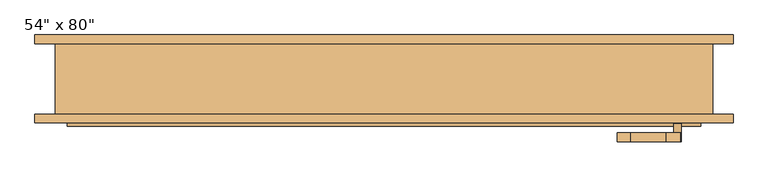
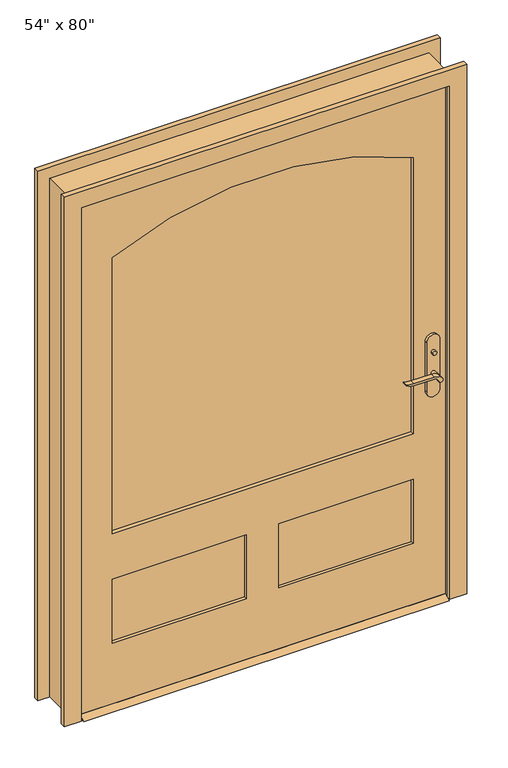
"""IFC4 building model written with IfcOpenShell, lengths in millimetres: door geometry."""

from ifc_helpers import new_model, si_unit, point, frame, frame_2d, origin, place, context, project, spatial, polyline, circle_curve, trimmed, segment, composite_curve, outline, extrude, faceted_brep, source, transform, mapped, element, save


def door_483975e0(model_context):
    return source(origin(), model_context, "Body", "SolidModel", [
        extrude(outline(polyline([(-38.1, 12.7), (-12.7, 0.0), (-98.425, 0.0), (-73.025, 12.7), (-38.1, 12.7)])), frame((-685.8, 0.0, 0.0), z_axis=(1.0, 0.0, 0.0), x_axis=(0.0, 1.0, 0.0)), (0.0, 0.0, 1.0), 1371.6),
        extrude(outline(polyline([(640.0, -18.1), (640.0, -28.1), (630.0, -28.1), (630.0, -18.1), (640.0, -18.1)])), frame((0.0, 0.0, 981.9), z_axis=(0.0, 0.0, 1.0), x_axis=(1.0, 0.0, 0.0)), (0.0, 0.0, 1.0), 30.0),
        extrude(outline(composite_curve([segment(trimmed(circle_curve(frame_2d((996.9, 635.0)), 8.0), [point((996.9, 627.0))], [point((996.9, 643.0))], False, "CARTESIAN"), True, "CONTINUOUS"), segment(trimmed(circle_curve(frame_2d((996.9, 635.0)), 8.0), [point((996.9, 643.0))], [point((996.9, 627.0))], False, "CARTESIAN"), True, "CONTINUOUS")], self_intersect=False)), frame((0.0, -93.025, 0.0), z_axis=(0.0, 1.0, 0.0), x_axis=(0.0, 0.0, 1.0)), (0.0, 0.0, 1.0), 10.0),
        extrude(outline(composite_curve([segment(trimmed(circle_curve(frame_2d((897.1555521, 611.3324871)), 37.2832219), [point((919.0523287, 641.5081363))], [point((934.4, 609.6325667))], False, "CARTESIAN"), True, "CONTINUOUS"), segment(polyline([(934.4, 609.6325667), (934.4, 533.3564091)]), True, "CONTINUOUS"), segment(trimmed(circle_curve(frame_2d((1017.6850638, 533.4227909)), 83.2850902), [point((934.4, 533.3564091))], [point((939.4, 505.0))], True, "CARTESIAN"), True, "CONTINUOUS"), segment(polyline([(939.4, 505.0), (936.6135558, 505.0)]), True, "CONTINUOUS"), segment(trimmed(circle_curve(frame_2d((986.6709207, 536.9396612)), 59.3791355), [point((936.6135558, 505.0))], [point((927.4, 533.3564091))], False, "CARTESIAN"), True, "CONTINUOUS"), segment(polyline([(927.4, 533.3564091), (927.4, 609.6138099)]), True, "CONTINUOUS"), segment(trimmed(circle_curve(frame_2d((909.2738613, 609.6138099)), 18.1261387), [point((927.4, 609.6138099))], [point((914.4, 627.0))], True, "CARTESIAN"), True, "CONTINUOUS"), segment(trimmed(circle_curve(frame_2d((914.4, 635.0)), 8.0), [point((914.4, 627.0))], [point((919.0523287, 641.5081363))], False, "CARTESIAN"), True, "CONTINUOUS")], self_intersect=False)), frame((0.0, 1.9, 0.0), z_axis=(0.0, 1.0, 0.0), x_axis=(0.0, 0.0, 1.0)), (0.0, 0.0, 1.0), 20.0),
        extrude(outline(composite_curve([segment(trimmed(circle_curve(frame_2d((914.4, 635.0)), 8.0), [point((914.3999903, 627.0))], [point((919.0523287, 641.5081363))], False, "CARTESIAN"), True, "CONTINUOUS"), segment(trimmed(circle_curve(frame_2d((897.1555521, 611.3324871)), 37.2832219), [point((919.0523287, 641.5081363))], [point((934.4, 609.6325667))], False, "CARTESIAN"), True, "CONTINUOUS"), segment(polyline([(934.4, 609.6325667), (934.4, 533.3564091)]), True, "CONTINUOUS"), segment(trimmed(circle_curve(frame_2d((1017.6850638, 533.4227909)), 83.2850902), [point((934.4, 533.3564091))], [point((939.4, 505.0))], True, "CARTESIAN"), True, "CONTINUOUS"), segment(polyline([(939.4, 505.0), (936.6135558, 505.0)]), True, "CONTINUOUS"), segment(trimmed(circle_curve(frame_2d((986.6709207, 536.9396612)), 59.3791355), [point((936.6135558, 505.0))], [point((927.4, 533.3564091))], False, "CARTESIAN"), True, "CONTINUOUS"), segment(polyline([(927.4, 533.3564091), (927.4, 609.6138122)]), True, "CONTINUOUS"), segment(trimmed(circle_curve(frame_2d((909.2738682, 609.6138122)), 18.1261318), [point((927.4, 609.6138122))], [point((914.3999903, 627.0))], True, "CARTESIAN"), True, "CONTINUOUS")], self_intersect=False)), frame((0.0, -133.025, 0.0), z_axis=(0.0, 1.0, 0.0), x_axis=(0.0, 0.0, 1.0)), (0.0, 0.0, 1.0), 20.0),
        extrude(outline(composite_curve([segment(trimmed(circle_curve(frame_2d((914.4, 635.0)), 8.0), [point((914.4, 627.0))], [point((914.4, 643.0))], False, "CARTESIAN"), True, "CONTINUOUS"), segment(trimmed(circle_curve(frame_2d((914.4, 635.0)), 8.0), [point((914.4, 643.0))], [point((914.4, 627.0))], False, "CARTESIAN"), True, "CONTINUOUS")], self_intersect=False)), frame((0.0, -28.1, 0.0), z_axis=(0.0, 1.0, 0.0), x_axis=(0.0, 0.0, 1.0)), (0.0, 0.0, 1.0), 30.0),
        extrude(outline(composite_curve([segment(trimmed(circle_curve(frame_2d((914.4, 635.0)), 8.0), [point((914.4, 627.0))], [point((914.4, 643.0))], False, "CARTESIAN"), True, "CONTINUOUS"), segment(trimmed(circle_curve(frame_2d((914.4, 635.0)), 8.0), [point((914.4, 643.0))], [point((914.4, 627.0))], False, "CARTESIAN"), True, "CONTINUOUS")], self_intersect=False)), frame((0.0, -113.025, 0.0), z_axis=(0.0, 1.0, 0.0), x_axis=(0.0, 0.0, 1.0)), (0.0, 0.0, 1.0), 30.0),
        extrude(outline(composite_curve([segment(polyline([(844.4, 660.0), (1039.4, 660.0)]), True, "CONTINUOUS"), segment(trimmed(circle_curve(frame_2d((1039.4, 635.0)), 25.0), [point((1039.4, 660.0))], [point((1039.4, 610.0))], False, "CARTESIAN"), True, "CONTINUOUS"), segment(polyline([(1039.4, 610.0), (844.4, 610.0)]), True, "CONTINUOUS"), segment(trimmed(circle_curve(frame_2d((844.4, 635.0)), 25.0), [point((844.4, 610.0))], [point((844.4, 660.0))], False, "CARTESIAN"), True, "CONTINUOUS")], self_intersect=False)), frame((0.0, -38.1, 0.0), z_axis=(0.0, 1.0, 0.0), x_axis=(0.0, 0.0, 1.0)), (0.0, 0.0, 1.0), 10.0),
        extrude(outline(composite_curve([segment(polyline([(844.4, 660.0), (1039.4, 660.0)]), True, "CONTINUOUS"), segment(trimmed(circle_curve(frame_2d((1039.4, 635.0)), 25.0), [point((1039.4, 660.0))], [point((1039.4, 610.0))], False, "CARTESIAN"), True, "CONTINUOUS"), segment(polyline([(1039.4, 610.0), (844.4, 610.0)]), True, "CONTINUOUS"), segment(trimmed(circle_curve(frame_2d((844.4, 635.0)), 25.0), [point((844.4, 610.0))], [point((844.4, 660.0))], False, "CARTESIAN"), True, "CONTINUOUS")], self_intersect=False)), frame((0.0, -83.025, 0.0), z_axis=(0.0, 1.0, 0.0), x_axis=(0.0, 0.0, 1.0)), (0.0, 0.0, 1.0), 10.0),
        extrude(outline(polyline([(2032.0, -685.8), (12.7, -685.8), (12.7, 685.8), (2032.0, 685.8), (2032.0, -685.8)]), holes=[composite_curve([segment(polyline([(688.975, -565.15), (1784.35, -565.15)]), True, "CONTINUOUS"), segment(trimmed(circle_curve(frame_2d((590.39125, 0.0)), 1320.95875), [point((1784.35, -565.15))], [point((1784.35, 565.15))], True, "CARTESIAN"), True, "CONTINUOUS"), segment(polyline([(1784.35, 565.15), (688.975, 565.15), (688.975, -565.15)]), True, "CONTINUOUS")], self_intersect=False), polyline([(508.0, -60.325), (254.0, -60.325), (254.0, -565.15), (508.0, -565.15), (508.0, -60.325)]), polyline([(508.0, 565.15), (254.0, 565.15), (254.0, 60.325), (508.0, 60.325), (508.0, 565.15)])]), frame((0.0, -73.025, 0.0), z_axis=(0.0, 1.0, 0.0), x_axis=(0.0, 0.0, 1.0)), (0.0, 0.0, 1.0), 34.925),
        faceted_brep([(711.2, -73.025, 0.0), (685.8, -73.025, 0.0), (685.8, -38.1, 0.0), (673.1, -38.1, 0.0), (673.1, -3.175, 0.0), (685.8, -3.175, 0.0), (685.8, 79.375, 0.0), (711.2, 79.375, 0.0), (711.2, 79.375, 2057.4), (711.2, -73.025, 2057.4), (685.8, 79.375, 2032.0), (-685.8, 79.375, 2032.0), (-685.8, 79.375, 0.0), (-711.2, 79.375, 0.0), (-711.2, 79.375, 2057.4), (685.8, -3.175, 2032.0), (673.1, -3.175, 2019.3), (-673.1, -3.175, 2019.3), (-673.1, -3.175, 0.0), (-685.8, -3.175, 0.0), (-685.8, -3.175, 2032.0), (673.1, -38.1, 2019.3), (685.8, -38.1, 2032.0), (-685.8, -38.1, 2032.0), (-685.8, -38.1, 0.0), (-673.1, -38.1, 0.0), (-673.1, -38.1, 2019.3), (685.8, -73.025, 2032.0), (-711.2, -73.025, 2057.4), (-711.2, -73.025, 0.0), (-685.8, -73.025, 0.0), (-685.8, -73.025, 2032.0)], [[[0, 1, 2, 3, 4, 5, 6, 7]], [[7, 8, 9, 0]], [[6, 10, 11, 12, 13, 14, 8, 7]], [[5, 15, 10, 6]], [[4, 16, 17, 18, 19, 20, 15, 5]], [[3, 21, 16, 4]], [[2, 22, 23, 24, 25, 26, 21, 3]], [[1, 27, 22, 2]], [[0, 9, 28, 29, 30, 31, 27, 1]], [[8, 14, 28, 9]], [[15, 20, 11, 10]], [[21, 26, 17, 16]], [[27, 31, 23, 22]], [[29, 13, 12, 19, 18, 25, 24, 30]], [[14, 13, 29, 28]], [[20, 19, 12, 11]], [[26, 25, 18, 17]], [[31, 30, 24, 23]]]),
        extrude(outline(polyline([(-60.325, -49.7416667), (-60.325, -61.3833333), (-565.15, -61.3833333), (-565.15, -49.7416667), (-60.325, -49.7416667)])), frame((0.0, 0.0, 254.0), z_axis=(0.0, 0.0, 1.0), x_axis=(1.0, 0.0, 0.0)), (0.0, 0.0, 1.0), 254.0),
        extrude(outline(polyline([(565.15, -49.7416667), (565.15, -61.3833333), (60.325, -61.3833333), (60.325, -49.7416667), (565.15, -49.7416667)])), frame((0.0, 0.0, 254.0), z_axis=(0.0, 0.0, 1.0), x_axis=(1.0, 0.0, 0.0)), (0.0, 0.0, 1.0), 254.0),
        extrude(outline(composite_curve([segment(polyline([(688.975, -565.15), (688.975, 565.15), (1784.35, 565.15)]), True, "CONTINUOUS"), segment(trimmed(circle_curve(frame_2d((590.39125, 0.0)), 1320.95875), [point((1784.35, 565.15))], [point((1784.35, -565.15))], False, "CARTESIAN"), True, "CONTINUOUS"), segment(polyline([(1784.35, -565.15), (688.975, -565.15)]), True, "CONTINUOUS")], self_intersect=False)), frame((0.0, -59.055, 0.0), z_axis=(0.0, 1.0, 0.0), x_axis=(0.0, 0.0, 1.0)), (0.0, 0.0, 1.0), 6.985),
        extrude(outline(polyline([(0.0, -692.15), (2038.35, -692.15), (2038.35, 692.15), (0.0, 692.15), (0.0, 755.65), (2101.85, 755.65), (2101.85, -755.65), (0.0, -755.65), (0.0, -692.15)])), frame((0.0, 79.375, 0.0), z_axis=(0.0, 1.0, 0.0), x_axis=(0.0, 0.0, 1.0)), (0.0, 0.0, 1.0), 19.05),
        extrude(outline(polyline([(0.0, -692.15), (2038.35, -692.15), (2038.35, 692.15), (0.0, 692.15), (0.0, 755.65), (2101.85, 755.65), (2101.85, -755.65), (0.0, -755.65), (0.0, -692.15)])), frame((0.0, -92.075, 0.0), z_axis=(0.0, 1.0, 0.0), x_axis=(0.0, 0.0, 1.0)), (0.0, 0.0, 1.0), 19.05),
    ])


if __name__ == "__main__":
    model = new_model("IFC4")
    model_context = context("Model", 3, world=origin())
    ifc_project = project(units=[si_unit("LENGTHUNIT", "METRE", prefix="MILLI")], contexts=[model_context])
    site = spatial("IfcSite", under=ifc_project)
    building = spatial("IfcBuilding", under=site)
    placement = place(None, origin())
    door_shape = door_483975e0(model_context)
    element("IfcDoor", 1, ObjectType="54\" x 80\"", at=placement, inside=building, context=model_context, shape_type="MappedRepresentation", body=[
        mapped(door_shape, transform((0.0, 0.0, 0.0), x_axis=(1.0, 0.0, 0.0), y_axis=(0.0, 1.0, 0.0), z_axis=(0.0, 0.0, 1.0))),
    ])
    save(model, "model.ifc")

# Revit data of these elements
# Type "54\" x 80\""
#   Type Mark = "8"
#   Assembly Code = "B2030100"
#   Analytic Construction = "French door, wood frame with single glass"
#   Threshold Offset [instance default] = 0' - 0 1/2"
#   Thickness = 0' - 1 3/8"
#   Thermal Resistance (R) = 1.0696 (h·ft²·°F)/BTU
#   Swing Angle [instance default] = 90.00°
#   Stiles = 0' - 4 3/4"
#   Rough Width = 4' - 8"
#   Rough Height = 6' - 9"
#   Radius = 4' - 4.00625"
#   Lock Rail = 0' - 7 1/8"
#   Height = 6' - 8"
#   Width = 4' - 6"
#   Heat Transfer Coefficient (U) = 0.9350 BTU/(h·ft²·°F)
#   Door Offset [instance default] = 0' - 0"
#   Bottom Rail = 0' - 9 1/2"
#   Threshold [instance default] = yes
#   Function = 1
#   Exterior Trim [instance default] = yes
#   Trim Material = Cherry
#   Threshold Material = Cherry
#   Panel Material = Cherry
#   Glazing = Glass
#   Frame Material = Cherry
#   Door Handle Material = Aluminum
#   Visual Light Transmittance = 0
#   Solar Heat Gain Coefficient = 0
#   Wall Closure = (empty or 0)
#   Construction Type = (empty or 0)
# Element 1 (IfcDoor, "54\" x 80\"")
#   Materials on its faces: "Cherry", "Aluminum", "Glass"
# Materials
#   "Cherry": class "Wood", colour RGB 226 177 128, transparency 0, Description = "Prunus Serotina", Cost = 0
#   "Glass": class "Glass", colour RGB 0 128 192, transparency 0.75, Description = "Soda Lime Glass", Cost = 0
#   "Aluminum": class "Metal", colour RGB 247 247 247, transparency 0, Description = "Aluminum 6061", Cost = 0
